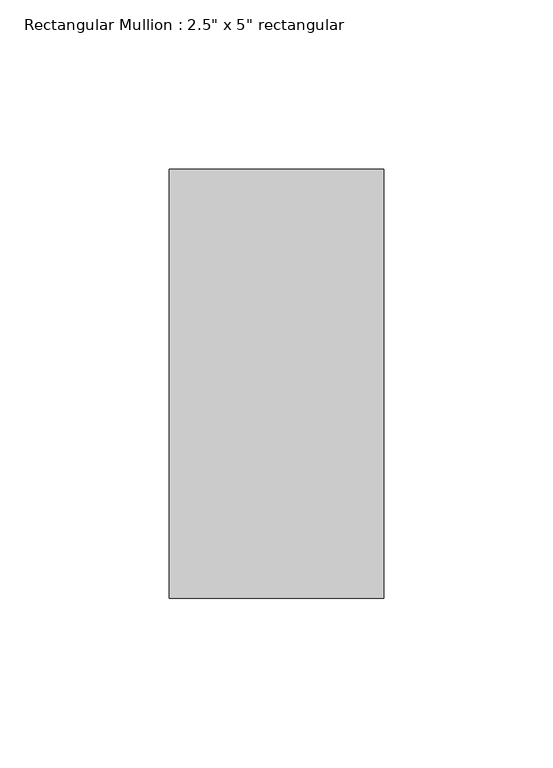
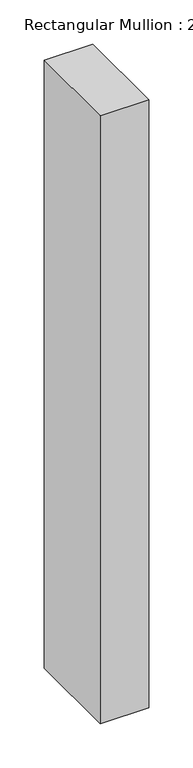
"""IFC4 building model written with IfcOpenShell, lengths in millimetres: member geometry."""

from ifc_helpers import new_model, si_unit, frame, origin, place, context, project, spatial, polyline, outline, extrude, source, transform, mapped, element, save


def member_9ef15e39(model_context):
    return source(origin(), model_context, "Body", "SweptSolid", [
        extrude(outline(polyline([(0.0, 63.5), (0.0, -63.5), (-63.5, -63.5), (-63.5, 63.5), (0.0, 63.5)])), frame((0.0, 0.0, -841.0108663), z_axis=(0.0, 0.0, 1.0), x_axis=(1.0, 0.0, 0.0)), (0.0, 0.0, 1.0), 841.0108663),
    ])


if __name__ == "__main__":
    model = new_model("IFC4")
    model_context = context("Model", 3, world=origin())
    ifc_project = project(units=[si_unit("LENGTHUNIT", "METRE", prefix="MILLI")], contexts=[model_context])
    site = spatial("IfcSite", under=ifc_project)
    building = spatial("IfcBuilding", under=site)
    placement = place(None, origin())
    member_shape = member_9ef15e39(model_context)
    element("IfcMember", 1, ObjectType="Rectangular Mullion : 2.5\" x 5\" rectangular", at=placement, inside=building, context=model_context, shape_type="MappedRepresentation", body=[
        mapped(member_shape, transform((0.0, 0.0, 0.0), x_axis=(1.0, 0.0, 0.0), y_axis=(0.0, 1.0, 0.0), z_axis=(0.0, 0.0, 1.0))),
    ])
    save(model, "model.ifc")

# Revit data of these elements
# Type "Rectangular Mullion : 2.5\" x 5\" rectangular"
#   built-in parameter 1007304 = 0.416667 (stored number, unit not read)
#   built-in parameter 1007301 = 0.104167 (stored number, unit not read)
#   built-in parameter 1007300 = 0.104167 (stored number, unit not read)
# Element 1 (IfcMember, "Rectangular Mullion : 2.5\" x 5\" rectangular")
#   Materials on its faces: "Aluminum"
# Materials
#   "Aluminum": class "Metal", colour RGB 247 247 247, transparency 0, Description = "Aluminum 6061", Cost = 0
